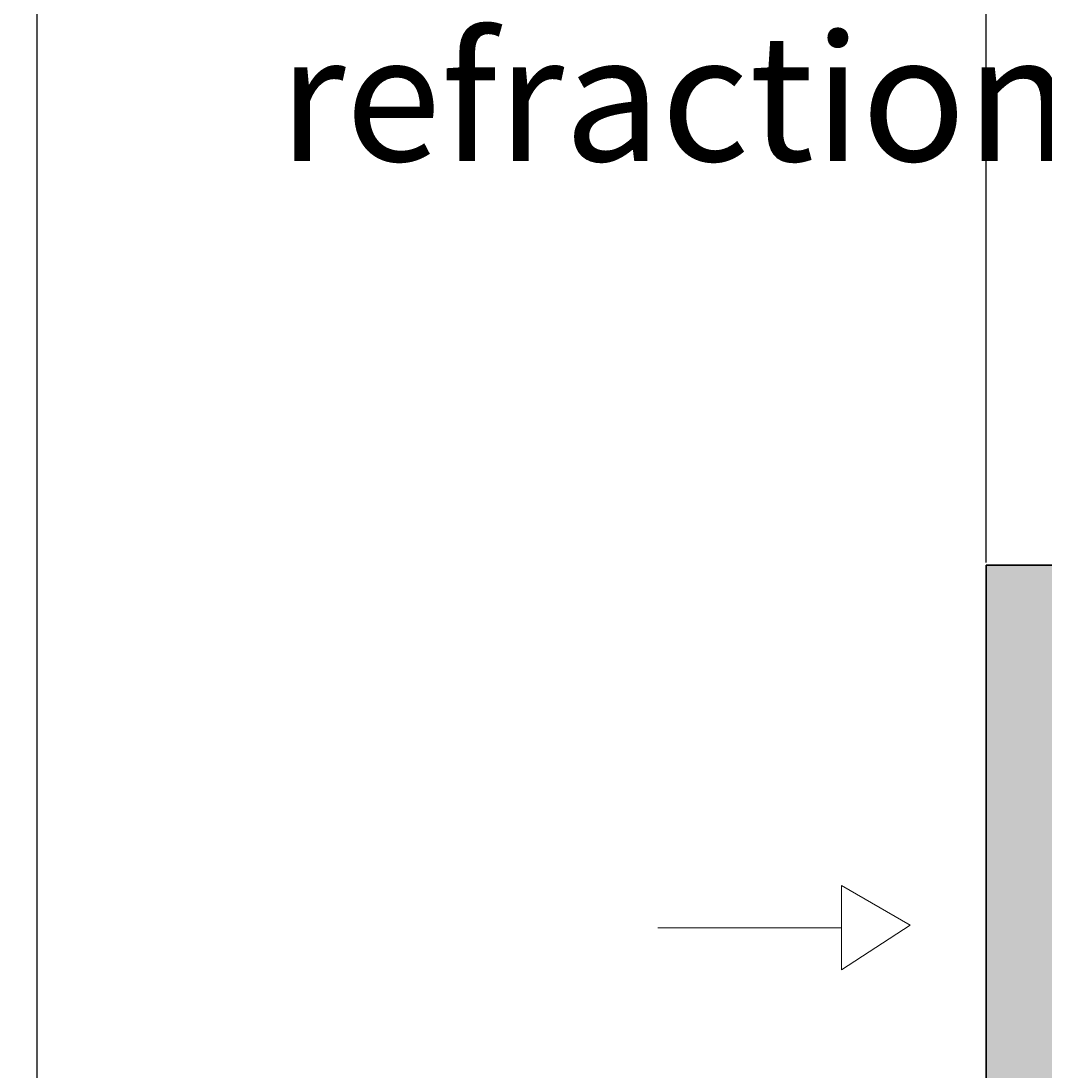
# Model space of a CAD drawing. Units: inches. Extents: x -1 to 292, y -3 to 199.
# Tile 6 of 52: x -1 to 23, y 77 to 101. Entities that reach past the tile are written whole.
import ezdxf

# ---------------------------------------------------------------- set-up
doc = ezdxf.new("R2010")
doc.units = ezdxf.units.IN
doc.header["$MEASUREMENT"] = 0
for name, color, linetype, lineweight in [('M-ANNO-SYMB', 1, 'Continuous', 18), ('M-ANNO-TEXT', 3, 'Continuous', 25), ('M-DIMS', 2, 'Continuous', 18), ('M-EQPM', 7, 'Continuous', 35), ('M-PATT', 8, 'Continuous', 13)]:
    doc.layers.add(name, color=color, linetype=linetype, lineweight=lineweight)
doc.styles.get("Standard").update_dxf_attribs({"font": 'arial.ttf'})
doc.dimstyles.get("Standard").update_dxf_attribs({"dimtxt": 0.18, "dimasz": 0.18, "dimexe": 0.18, "dimexo": 0.0625, "dimgap": 0.09, "dimtad": 0, "dimtih": 1, "dimtoh": 1, "dimdec": 4, "dimzin": 0, "dimdsep": 46, "dimtxsty": 'Standard', "dimcen": 0.09, "dimadec": 0, "dimazin": 0, "dimtfac": 1, "dimtdec": 4, "dimtofl": 0, "dimtmove": 0, "dimatfit": 3, "dimfxl": 1, "dimtolj": 1, "dimtzin": 0, "dimarcsym": 0})

# ---------------------------------------------------------------- blocks, each defined once
blk = doc.blocks.new('FLOW-ARROW-GAS')
for p, q in [((201.507, 38.14), (201.507, 36.14)), ((201.507, 38.14), (203.137, 37.199)), ((201.507, 37.14), (197.151, 37.14)), ((201.507, 36.14), (203.137, 37.199))]:
    blk.add_line(p, q)
blk = doc.blocks.new('DUCT-FLANGE')
for p, q in [((0, 34), (0, 0)), ((0, 34), (2.089, 34)), ((2.089, 34), (2.089, 0)), ((0, 0), (2.089, 0))]:
    blk.add_line(p, q)
blk = doc.blocks.new('*D8')
at = {"layer": 'Defpoints', "color": 0, "transparency": 16777216}
for p in [(-0.662, 126.765), (111.488, 126.765), (69.013, 25.514)]:
    blk.add_point(p, dxfattribs=at)
at = {"layer": 'M-DIMS', "color": 0, "lineweight": -2, "transparency": 16777216}
for p, q in [((111.426, 126.765), (-0.842, 126.765)), ((-0.662, 126.585), (-0.662, 76.321)), ((-0.662, 25.694), (-0.662, 75.958)), ((68.951, 25.514), (-0.842, 25.514))]:
    blk.add_line(p, q, dxfattribs=at)
at = {"layer": 'M-DIMS', "color": 0, "transparency": 16777216}
for points in [[(-0.692, 126.585), (-0.632, 126.585), (-0.662, 126.765)], [(-0.692, 25.694), (-0.632, 25.694), (-0.662, 25.514)]]:
    blk.add_solid(points, dxfattribs=at)
at = {"layer": 'M-DIMS', "color": 0, "transparency": 16777216, "insert": (-0.662, 76.14), "char_height": 0.18, "attachment_point": 5}
blk.add_mtext('\\A1;101.25', dxfattribs=at)
blk = doc.blocks.new('*D14')
at = {"layer": 'Defpoints', "color": 0, "transparency": 16777216}
for p in [(21.861, 88.582), (21.861, 54.582), (36.461, 54.582)]:
    blk.add_point(p, dxfattribs=at)
at = {"layer": 'M-DIMS', "color": 0, "lineweight": -2, "transparency": 16777216}
for p, q in [((21.924, 88.582), (36.641, 88.582)), ((36.461, 88.402), (36.461, 71.764)), ((36.461, 54.762), (36.461, 71.4)), ((21.924, 54.582), (36.641, 54.582))]:
    blk.add_line(p, q, dxfattribs=at)
at = {"layer": 'M-DIMS', "color": 0, "transparency": 16777216}
for points in [[(36.431, 88.402), (36.491, 88.402), (36.461, 88.582)], [(36.431, 54.762), (36.491, 54.762), (36.461, 54.582)]]:
    blk.add_solid(points, dxfattribs=at)
at = {"layer": 'M-DIMS', "color": 0, "transparency": 16777216, "insert": (36.461, 71.582), "char_height": 0.18, "attachment_point": 5}
blk.add_mtext('\\A1;34', dxfattribs=at)
blk = doc.blocks.new('*D15')
at = {"layer": 'Defpoints', "color": 0, "transparency": 16777216}
for p in [(23.95, 174.363), (21.861, 88.582), (23.95, 88.582)]:
    blk.add_point(p, dxfattribs=at)
at = {"layer": 'M-DIMS', "color": 0, "lineweight": -2, "transparency": 16777216}
for p, q in [((21.861, 88.645), (21.861, 174.543)), ((23.95, 88.645), (23.95, 174.543)), ((22.041, 174.363), (22.51, 174.363)), ((23.77, 174.363), (23.301, 174.363))]:
    blk.add_line(p, q, dxfattribs=at)
at = {"layer": 'M-DIMS', "color": 0, "transparency": 16777216}
for points in [[(22.041, 174.393), (22.041, 174.333), (21.861, 174.363)], [(23.77, 174.393), (23.77, 174.333), (23.95, 174.363)]]:
    blk.add_solid(points, dxfattribs=at)
at = {"layer": 'M-DIMS', "color": 0, "transparency": 16777216, "insert": (22.906, 174.363), "char_height": 0.18, "attachment_point": 5}
blk.add_mtext('\\A1;2.089', dxfattribs=at)

msp = doc.modelspace()

# ---------------------------------------------------------------- hatches: boundary and pattern name
at = {"layer": 'M-PATT'}
h = msp.add_hatch(color=256, dxfattribs=at)
h.set_gradient(color1=(76, 38, 47), color2=(76, 38, 47), tint=1, name='CYLINDER')
h.paths.add_polyline_path([(40.8628, 91.6478), (40.3591, 92.5203), (23.9502, 85.5552), (23.9502, 84.4688)])
h.paths.add_polyline_path([(52.8586, 93.6403), (42.9977, 93.6403), (40.3591, 92.5203), (40.8628, 91.6478), (43.2011, 92.6403), (54.4604, 92.6403, -0.0601508)])
h.paths.add_polyline_path([(23.9502, 88.5821), (21.8612, 88.5821), (21.8612, 54.5821), (23.9502, 54.5821)])
h.paths.add_polyline_path([(23.9502, 58.376), (23.9502, 57.2213), (42.9332, 46.2615), (50.4659, 46.2615, -0.0351813), (50.9409, 47.2615), (43.2011, 47.2615)])
h.paths.add_polyline_path([(179.5897, 93.6403), (174.1181, 93.6403, -0.0601508), (172.5163, 92.6403), (179.5897, 92.6403)])
h.paths.add_polyline_path([(183.979, 93.6403), (181.5897, 93.6403), (181.5897, 92.6403), (183.7755, 92.6403), (203.0265, 84.4688), (203.0265, 85.5552)])
h.paths.add_polyline_path([(205.1155, 88.5821), (203.0265, 88.5821), (203.0265, 54.5821), (205.1155, 54.5821)])
h.paths.add_polyline_path([(203.0265, 57.2213), (203.0265, 58.376), (183.7755, 47.2615), (181.5897, 47.2615), (181.5897, 46.2615), (184.0435, 46.2615)])
h.paths.add_polyline_path([(179.5897, 47.2615), (176.0358, 47.2615, -0.0351813), (176.5107, 46.2615), (179.5897, 46.2615)])

# ---------------------------------------------------------------- block references
at = {"layer": 'M-ANNO-SYMB'}
msp.add_blockref('FLOW-ARROW-GAS', (-183.0766, 42.8359), dxfattribs=at)
at = {"layer": 'M-EQPM'}
msp.add_blockref('DUCT-FLANGE', (21.861, 54.582), dxfattribs=at)

# ---------------------------------------------------------------- texts
at = {"layer": 'M-ANNO-TEXT', "insert": (5.0709, 101.1707), "char_height": 3, "attachment_point": 1}
msp.add_mtext_dynamic_manual_height_columns('refraction lining', width=47.899539, gutter_width=1, heights=[0], dxfattribs=at)

# ---------------------------------------------------------------- dimensions: what is measured, and where the dimension line sits
at = {"layer": 'M-DIMS'}
dim = msp.add_linear_dim(base=(23.9502, 174.3627), p1=(21.8612, 88.5821), p2=(23.9502, 88.5821), dimstyle='Standard', override={"dimdec": 3, "dimlfac": 1, "dimrnd": 0, "dimzin": 0, "dimdsep": 46, "dimlunit": 2}, dxfattribs=at)
dim.commit()
dim.dimension.update_dxf_attribs({"geometry": '*D15', "text_midpoint": (22.9057, 174.3627)})
for base, p1, p2, angle, override, picture, middle in [((-0.6625, 126.765), (69.013, 25.5141), (111.4883, 126.765), 90, {"dimdec": 2, "dimlfac": 1, "dimrnd": 0, "dimzin": 0, "dimdsep": 46, "dimlunit": 2}, '*D8', (-0.6625, 76.1396)), ((36.4612, 54.5821), (21.8612, 88.5821), (21.8612, 54.5821), 270, {"dimdec": 0, "dimlfac": 1, "dimrnd": 0, "dimzin": 0, "dimdsep": 46, "dimlunit": 2}, '*D14', (36.4612, 71.5821))]:
    dim = msp.add_linear_dim(base=base, p1=p1, p2=p2, angle=angle, dimstyle='Standard', override=override, dxfattribs=at)
    dim.commit()
    dim.dimension.update_dxf_attribs({"geometry": picture, "text_midpoint": middle})

doc.saveas('drawing.dxf')
